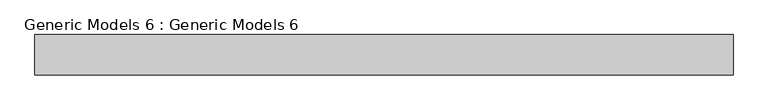
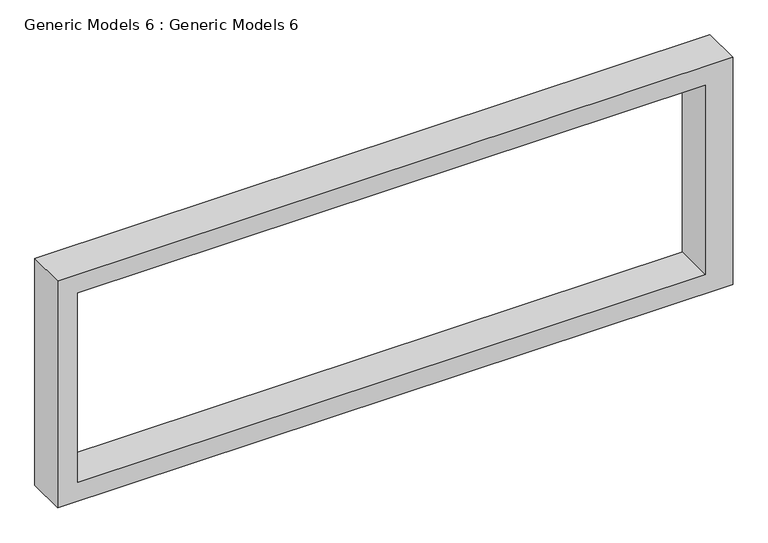
"""IFC4 building model written with IfcOpenShell, lengths in millimetres: proxy geometry, Generic Models 6 : Generic Models 6."""

from ifc_helpers import new_model, si_unit, frame, origin, place, context, project, spatial, polyline, outline, extrude, source, transform, mapped, element, save


def generic_models_6_generic_models_6_b3d137af(model_context):
    return source(origin(), model_context, "Body", "SweptSolid", [
        extrude(outline(polyline([(7010.4, 4189.5719693), (7010.4, -6097.4280307), (3352.8, -6097.4280307), (3352.8, 4189.5719693), (7010.4, 4189.5719693)]), holes=[polyline([(6705.6, 3770.4719693), (3657.6, 3770.4719693), (3657.6, -5792.6280307), (6705.6, -5792.6280307), (6705.6, 3770.4719693)])]), frame((0.0, -6514.0041706, 0.0), z_axis=(0.0, 1.0, 0.0), x_axis=(0.0, 0.0, 1.0)), (0.0, 0.0, 1.0), 595.8682958),
    ])


if __name__ == "__main__":
    model = new_model("IFC4")
    model_context = context("Model", 3, world=origin())
    ifc_project = project(units=[si_unit("LENGTHUNIT", "METRE", prefix="MILLI")], contexts=[model_context])
    site = spatial("IfcSite", under=ifc_project)
    building = spatial("IfcBuilding", under=site)
    placement = place(None, origin())
    generic_models_6_generic_models_6_shape = generic_models_6_generic_models_6_b3d137af(model_context)
    element("IfcBuildingElementProxy", 1, Name="Generic Models 6 : Generic Models 6", ObjectType="Generic Models 6 : Generic Models 6", at=placement, inside=building, context=model_context, shape_type="MappedRepresentation", body=[
        mapped(generic_models_6_generic_models_6_shape, transform((0.0, 0.0, 0.0), x_axis=(1.0, 0.0, 0.0), y_axis=(0.0, 1.0, 0.0), z_axis=(0.0, 0.0, 1.0))),
    ])
    save(model, "model.ifc")

# Revit data of these elements
# Element 1 (IfcBuildingElementProxy, "Generic Models 6 : Generic Models 6")
#   Materials on its faces: "chocolate brown"
# Materials
#   "chocolate brown": class "Generic", colour RGB 120 120 120, transparency 0, Cost = 0
